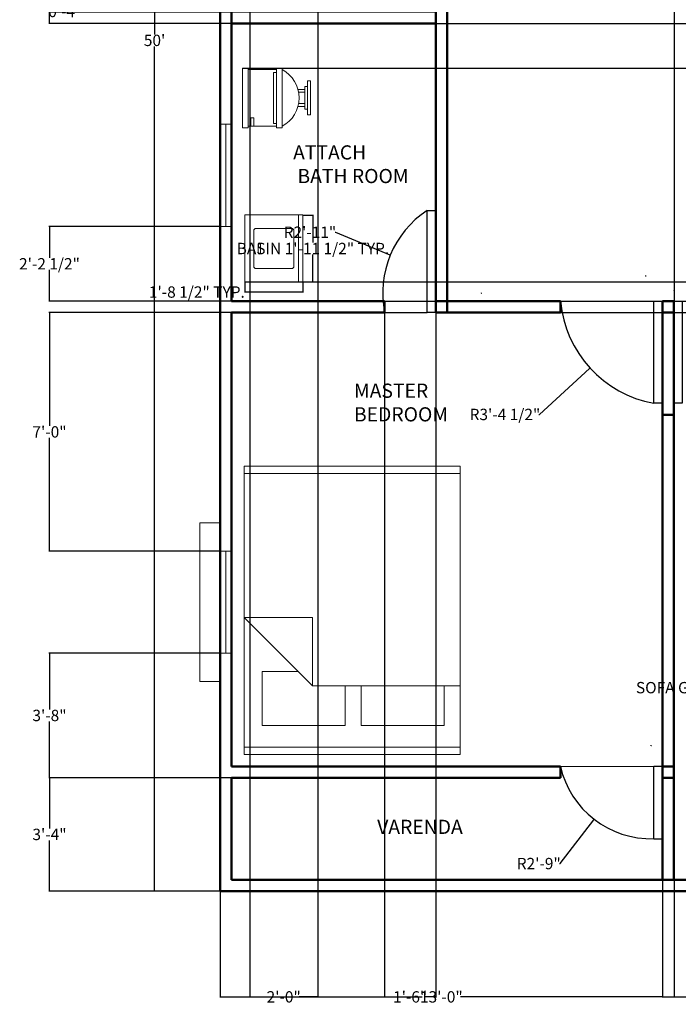
# Model space of a CAD drawing. Units: inches. Extents: x 749 to 1356, y 222 to 907.
# Tile 1 of 4: x 750 to 982, y 222 to 570. Entities that reach past the tile are written whole.
import ezdxf

# ---------------------------------------------------------------- set-up
doc = ezdxf.new("R2010")
doc.units = ezdxf.units.IN
doc.header["$MEASUREMENT"] = 0
for name, color, linetype, lineweight in [('A-ANNO-DIMS', 30, 'Continuous', 18), ('A-AREA-IDEN', 6, 'Continuous', 25), ('A-FLOR-FIXT', 9, 'Continuous', 18), ('A-GLAZ', 4, 'Continuous', 20), ('A-WALL', 7, 'Continuous', 50), ('DOOR', 4, 'Continuous', 25), ('FURNITURE', 32, 'Continuous', 18)]:
    doc.layers.add(name, color=color, linetype=linetype, lineweight=lineweight)
doc.styles.get("Standard").update_dxf_attribs({"font": 'arial.ttf'})
doc.dimstyles.get("Standard").update_dxf_attribs({"dimtxt": 4, "dimasz": 0.18, "dimexe": 0.18, "dimexo": 0.0625, "dimgap": 0.09, "dimtad": 0, "dimtih": 1, "dimtoh": 1, "dimdec": 0, "dimrnd": 6, "dimzin": 0, "dimdsep": 46, "dimlunit": 3, "dimtxsty": 'Standard', "dimcen": 0.09, "dimadec": 0, "dimazin": 0, "dimtfac": 1, "dimtdec": 0, "dimtofl": 0, "dimtmove": 0, "dimatfit": 3, "dimfxl": 1, "dimtolj": 1, "dimtzin": 0, "dimarcsym": 0})

# ---------------------------------------------------------------- blocks, each defined once
blk = doc.blocks.new('Toilet - Imperial')
for p, q in [((-10, 22), (-10, 12)), ((-10, 21), (-7, 21)), ((-7, 21), (-7, 20)), ((10, 12), (10, 22)), ((-7, 20), (-10, 20)), ((10.5, 12), (-10.5, 12)), ((-10.5, 10), (-10.5, 12)), ((9, 13), (-9, 13)), ((-9, 13), (-9, 12)), ((9, 12), (9, 13)), ((10.5, 12), (10.5, 10)), ((10.5, 10), (-10.5, 10)), ((-3, 4.4065), (-3, 2)), ((-2, 2), (-2, 4.1658)), ((2, 4.1658), (2, 2)), ((3, 2), (3, 4.4065)), ((4, 2), (-4, 2)), ((-4, 2), (-4, 1)), ((4, 1), (4, 2))]:
    blk.add_line(p, q)
for points in [[(10.5, 22), (10.5, 24), (-10.5, 24), (-10.5, 22)], [(6, 0), (6, 1), (-6, 1), (-6, 0)]]:
    blk.add_lwpolyline(points, close=True)
blk.add_arc((0, 15.3333), 11.3333, 208.0725, 331.9275)
blk = doc.blocks.new('QUEEN-00')
for p, q in [((-0.8475, -0.7751), (-0.8475, 0.7489)), ((0.6511, 0.7489), (0.6511, -0.2925)), ((1.0829, 0.7489), (1.0829, -0.7751)), ((0.9305, 0.6346), (0.6511, 0.6346)), ((0.9305, 0.0504), (0.9305, 0.6346)), ((0.6511, 0.0504), (0.9305, 0.0504)), ((0.9305, -0.0639), (0.6511, -0.0639)), ((0.9305, -0.6481), (0.9305, -0.0639)), ((0.1685, -0.7751), (0.6511, -0.2925)), ((0.1685, -0.2925), (0.1685, -0.7751)), ((0.6511, -0.2925), (0.1685, -0.2925)), ((0.5495, -0.3941), (0.5495, -0.6481)), ((0.5495, -0.6481), (0.9305, -0.6481))]:
    blk.add_line(p, q)
blk.add_lwpolyline([(-0.8983, -0.7751), (-0.8983, 0.7489), (1.1337, 0.7489), (1.1337, -0.7751)], close=True)
blk = doc.blocks.new('LAVAD-01')
for p, q in [((-0.322, 0.358), (-0.322, -0.392)), ((0.328, 0.358), (-0.322, 0.358)), ((-0.272, 0.358), (-0.272, -0.392)), ((0.328, -0.392), (0.328, 0.358)), ((-0.222, 0.183), (-0.222, -0.217)), ((0.203, 0.208), (-0.197, 0.208)), ((0.228, -0.217), (0.228, 0.183)), ((0.153, 0.033), (0.153, -0.067)), ((0.165, 0.046), (0.165, 0.046)), ((0.178, -0.067), (0.178, 0.033)), ((0.165, -0.079), (0.165, -0.079)), ((-0.197, -0.242), (0.203, -0.242)), ((-0.322, -0.392), (0.328, -0.392))]:
    blk.add_line(p, q)
for centre, radius, start, end in [((-0.197, 0.183), 0.025, 90, 180), ((0.203, 0.183), 0.025, 0, 90), ((0.165, 0.033), 0.0125, 90, 180), ((0.165, 0.033), 0.0125, 0, 90), ((0.165, -0.067), 0.0125, 180, 270), ((0.165, -0.067), 0.0125, 270, 360), ((-0.197, -0.217), 0.025, 180, 270), ((0.203, -0.217), 0.025, 270, 360)]:
    blk.add_arc(centre, radius, start, end)
blk = doc.blocks.new('*D130')
at = {"layer": 'A-ANNO-DIMS', "color": 0, "lineweight": -2, "transparency": 16777216}
for p, q in [((820.81, 862.27), (797.55, 862.27)), ((797.73, 862.09), (797.73, 564.4)), ((797.73, 262.45), (797.73, 560.13)), ((820.81, 262.27), (797.55, 262.27))]:
    blk.add_line(p, q, dxfattribs=at)
at = {"layer": 'A-ANNO-DIMS', "color": 0, "transparency": 16777216}
for points in [[(797.7, 862.09), (797.76, 862.09), (797.73, 862.27)], [(797.7, 262.45), (797.76, 262.45), (797.73, 262.27)]]:
    blk.add_solid(points, dxfattribs=at)
at = {"layer": 'Defpoints', "color": 0, "transparency": 16777216}
for p in [(820.88, 862.27), (797.73, 262.27), (820.88, 262.27)]:
    blk.add_point(p, dxfattribs=at)
at = {"layer": 'A-ANNO-DIMS', "color": 0, "transparency": 16777216, "insert": (797.73, 562.27), "char_height": 4, "attachment_point": 5}
blk.add_mtext("\\A1;50'", dxfattribs=at)
blk = doc.blocks.new('WIN-36IN')
blk.add_lwpolyline([(0, 0), (0, 36), (4, 36), (4, 0)], close=True)
blk.add_lwpolyline([(4, 0), (2.02, 0), (2.02, 36)])
blk = doc.blocks.new('DOOR-LEAF-36IN')
blk.add_lwpolyline([(0, 3), (36, 3), (36, 0), (0, 0)], close=True)
blk = doc.blocks.new('*D143')
at = {"layer": 'A-ANNO-DIMS', "color": 0, "lineweight": -2, "transparency": 16777216}
for p, q in [((850.11, 500.69), (853.77, 500.69)), ((853.59, 500.51), (853.59, 491.04)), ((853.59, 477.25), (853.59, 486.72)), ((850.11, 477.07), (853.77, 477.07))]:
    blk.add_line(p, q, dxfattribs=at)
at = {"layer": 'A-ANNO-DIMS', "color": 0, "transparency": 16777216}
for points in [[(853.56, 500.51), (853.62, 500.51), (853.59, 500.69)], [(853.56, 477.25), (853.62, 477.25), (853.59, 477.07)]]:
    blk.add_solid(points, dxfattribs=at)
at = {"layer": 'Defpoints', "color": 0, "transparency": 16777216}
for p in [(850.05, 500.69), (850.05, 477.07), (853.59, 477.07)]:
    blk.add_point(p, dxfattribs=at)
at = {"layer": 'A-ANNO-DIMS', "color": 0, "transparency": 16777216, "insert": (853.59, 488.88), "char_height": 4, "attachment_point": 5}
blk.add_mtext('\\A1;BASIN 1\'-11 1/2" TYP.', dxfattribs=at)
blk = doc.blocks.new('*D144')
at = {"layer": 'A-ANNO-DIMS', "color": 0, "lineweight": -2, "transparency": 16777216}
for p, q in [((829.57, 477.01), (829.57, 473.35)), ((850.05, 477.01), (850.05, 473.35)), ((829.57, 473.53), (829.39, 473.53)), ((849.87, 473.53), (829.75, 473.53))]:
    blk.add_line(p, q, dxfattribs=at)
at = {"layer": 'A-ANNO-DIMS', "color": 0, "transparency": 16777216}
for points in [[(829.75, 473.56), (829.75, 473.5), (829.57, 473.53)], [(849.87, 473.56), (849.87, 473.5), (850.05, 473.53)]]:
    blk.add_solid(points, dxfattribs=at)
at = {"layer": 'Defpoints', "color": 0, "transparency": 16777216}
for p in [(829.57, 477.07), (850.05, 477.07), (829.57, 473.53)]:
    blk.add_point(p, dxfattribs=at)
at = {"layer": 'A-ANNO-DIMS', "color": 0, "transparency": 16777216, "insert": (812.64, 473.53), "char_height": 4, "attachment_point": 5}
blk.add_mtext('\\A1;1\'-8 1/2" TYP.', dxfattribs=at)
blk = doc.blocks.new('*D153')
at = {"layer": 'A-ANNO-DIMS', "color": 0, "lineweight": -2, "transparency": 16777216}
for p, q in [((1011.97, 388.69), (995.45, 388.69)), ((995.63, 388.51), (995.63, 336.18)), ((995.63, 279.54), (995.63, 331.87)), ((1011.97, 279.36), (995.45, 279.36))]:
    blk.add_line(p, q, dxfattribs=at)
at = {"layer": 'A-ANNO-DIMS', "color": 0, "transparency": 16777216}
for points in [[(995.6, 388.51), (995.66, 388.51), (995.63, 388.69)], [(995.6, 279.54), (995.66, 279.54), (995.63, 279.36)]]:
    blk.add_solid(points, dxfattribs=at)
at = {"layer": 'Defpoints', "color": 0, "transparency": 16777216}
for p in [(1012.03, 388.69), (995.63, 279.36), (1012.03, 279.36)]:
    blk.add_point(p, dxfattribs=at)
at = {"layer": 'A-ANNO-DIMS', "color": 0, "transparency": 16777216, "insert": (995.63, 334.02), "char_height": 4, "attachment_point": 5}
blk.add_mtext('\\A1;SOFA GROUP 9\'-1 1/2"', dxfattribs=at)
blk = doc.blocks.new('*D155')
at = {"layer": 'A-ANNO-DIMS', "color": 0, "lineweight": -2, "transparency": 16777216}
for p, q in [((976.88, 266.2), (976.88, 224.8)), ((820.88, 262.2), (820.88, 224.8)), ((821.06, 224.98), (892.1, 224.98)), ((976.7, 224.98), (905.65, 224.98))]:
    blk.add_line(p, q, dxfattribs=at)
at = {"layer": 'A-ANNO-DIMS', "color": 0, "transparency": 16777216}
for points in [[(821.06, 225.01), (821.06, 224.95), (820.88, 224.98)], [(976.7, 225.01), (976.7, 224.95), (976.88, 224.98)]]:
    blk.add_solid(points, dxfattribs=at)
at = {"layer": 'Defpoints', "color": 0, "transparency": 16777216}
for p in [(976.88, 266.27), (820.88, 262.27), (976.88, 224.98)]:
    blk.add_point(p, dxfattribs=at)
at = {"layer": 'A-ANNO-DIMS', "color": 0, "transparency": 16777216, "insert": (898.88, 224.98), "char_height": 4, "attachment_point": 5}
blk.add_mtext('\\A1;13\'-0"', dxfattribs=at)
blk = doc.blocks.new('*D156')
at = {"layer": 'A-ANNO-DIMS', "color": 0, "lineweight": -2, "transparency": 16777216}
for p, q in [((976.88, 266.2), (976.88, 224.8)), ((1027.01, 266.19), (1027.01, 224.8)), ((977.06, 224.98), (996.46, 224.98)), ((1026.83, 224.98), (1007.43, 224.98))]:
    blk.add_line(p, q, dxfattribs=at)
at = {"layer": 'A-ANNO-DIMS', "color": 0, "transparency": 16777216}
for points in [[(977.06, 225.01), (977.06, 224.95), (976.88, 224.98)], [(1026.83, 225.01), (1026.83, 224.95), (1027.01, 224.98)]]:
    blk.add_solid(points, dxfattribs=at)
at = {"layer": 'Defpoints', "color": 0, "transparency": 16777216}
for p in [(976.88, 266.27), (1027.01, 266.25), (1027.01, 224.98)]:
    blk.add_point(p, dxfattribs=at)
at = {"layer": 'A-ANNO-DIMS', "color": 0, "transparency": 16777216, "insert": (1001.95, 224.98), "char_height": 4, "attachment_point": 5}
blk.add_mtext('\\A1;4\'-2"', dxfattribs=at)
blk = doc.blocks.new('*D159')
at = {"layer": 'A-ANNO-DIMS', "color": 0, "lineweight": -2, "transparency": 16777216}
for p, q in [((824.81, 302.27), (760.48, 302.27)), ((760.66, 302.09), (760.66, 284.4)), ((760.66, 262.45), (760.66, 280.13)), ((820.81, 262.27), (760.48, 262.27))]:
    blk.add_line(p, q, dxfattribs=at)
at = {"layer": 'A-ANNO-DIMS', "color": 0, "transparency": 16777216}
for points in [[(760.63, 302.09), (760.69, 302.09), (760.66, 302.27)], [(760.63, 262.45), (760.69, 262.45), (760.66, 262.27)]]:
    blk.add_solid(points, dxfattribs=at)
at = {"layer": 'Defpoints', "color": 0, "transparency": 16777216}
for p in [(760.66, 302.27), (824.88, 302.27), (820.88, 262.27)]:
    blk.add_point(p, dxfattribs=at)
at = {"layer": 'A-ANNO-DIMS', "color": 0, "transparency": 16777216, "insert": (760.66, 282.27), "char_height": 4, "attachment_point": 5}
blk.add_mtext('\\A1;3\'-4"', dxfattribs=at)
blk = doc.blocks.new('*D160')
at = {"layer": 'A-ANNO-DIMS', "color": 0, "lineweight": -2, "transparency": 16777216}
for p, q in [((820.79, 346.16), (760.48, 346.16)), ((760.66, 345.98), (760.66, 326.35)), ((760.66, 302.45), (760.66, 322.08)), ((824.81, 302.27), (760.48, 302.27))]:
    blk.add_line(p, q, dxfattribs=at)
at = {"layer": 'A-ANNO-DIMS', "color": 0, "transparency": 16777216}
for points in [[(760.63, 345.98), (760.69, 345.98), (760.66, 346.16)], [(760.63, 302.45), (760.69, 302.45), (760.66, 302.27)]]:
    blk.add_solid(points, dxfattribs=at)
at = {"layer": 'Defpoints', "color": 0, "transparency": 16777216}
for p in [(760.66, 346.16), (820.85, 346.16), (824.88, 302.27)]:
    blk.add_point(p, dxfattribs=at)
at = {"layer": 'A-ANNO-DIMS', "color": 0, "transparency": 16777216, "insert": (760.66, 324.21), "char_height": 4, "attachment_point": 5}
blk.add_mtext('\\A1;3\'-8"', dxfattribs=at)
blk = doc.blocks.new('*D161')
at = {"layer": 'A-ANNO-DIMS', "color": 0, "lineweight": -2, "transparency": 16777216}
for p, q in [((824.81, 466.27), (760.48, 466.27)), ((760.66, 466.09), (760.66, 426.35)), ((760.66, 382.34), (760.66, 422.08)), ((820.79, 382.16), (760.48, 382.16))]:
    blk.add_line(p, q, dxfattribs=at)
at = {"layer": 'A-ANNO-DIMS', "color": 0, "transparency": 16777216}
for points in [[(760.63, 466.09), (760.69, 466.09), (760.66, 466.27)], [(760.63, 382.34), (760.69, 382.34), (760.66, 382.16)]]:
    blk.add_solid(points, dxfattribs=at)
at = {"layer": 'Defpoints', "color": 0, "transparency": 16777216}
for p in [(760.66, 466.27), (824.88, 466.27), (820.85, 382.16)]:
    blk.add_point(p, dxfattribs=at)
at = {"layer": 'A-ANNO-DIMS', "color": 0, "transparency": 16777216, "insert": (760.66, 424.21), "char_height": 4, "attachment_point": 5}
blk.add_mtext('\\A1;7\'-0"', dxfattribs=at)
blk = doc.blocks.new('*D170')
at = {"layer": 'A-ANNO-DIMS', "color": 0, "lineweight": -2, "transparency": 16777216}
for p, q in [((820.74, 496.69), (760.48, 496.69)), ((760.66, 496.51), (760.66, 485.63)), ((760.66, 470.45), (760.66, 481.32)), ((824.81, 470.27), (760.48, 470.27))]:
    blk.add_line(p, q, dxfattribs=at)
at = {"layer": 'A-ANNO-DIMS', "color": 0, "transparency": 16777216}
for points in [[(760.63, 496.51), (760.69, 496.51), (760.66, 496.69)], [(760.63, 470.45), (760.69, 470.45), (760.66, 470.27)]]:
    blk.add_solid(points, dxfattribs=at)
at = {"layer": 'Defpoints', "color": 0, "transparency": 16777216}
for p in [(760.66, 496.69), (820.8, 496.69), (824.88, 470.27)]:
    blk.add_point(p, dxfattribs=at)
at = {"layer": 'A-ANNO-DIMS', "color": 0, "transparency": 16777216, "insert": (760.66, 483.48), "char_height": 4, "attachment_point": 5}
blk.add_mtext('\\A1;2\'-2 1/2"', dxfattribs=at)
blk = doc.blocks.new('*D173')
at = {"layer": 'A-ANNO-DIMS', "color": 0, "lineweight": -2, "transparency": 16777216}
for p, q in [((896.94, 568.27), (1340.58, 568.27)), ((1340.4, 568.09), (1340.4, 519.4)), ((1340.4, 466.45), (1340.4, 515.13)), ((900.94, 466.27), (1340.58, 466.27))]:
    blk.add_line(p, q, dxfattribs=at)
at = {"layer": 'A-ANNO-DIMS', "color": 0, "transparency": 16777216}
for points in [[(1340.37, 568.09), (1340.43, 568.09), (1340.4, 568.27)], [(1340.37, 466.45), (1340.43, 466.45), (1340.4, 466.27)]]:
    blk.add_solid(points, dxfattribs=at)
at = {"layer": 'Defpoints', "color": 0, "transparency": 16777216}
for p in [(896.88, 568.27), (1340.4, 568.27), (900.88, 466.27)]:
    blk.add_point(p, dxfattribs=at)
at = {"layer": 'A-ANNO-DIMS', "color": 0, "transparency": 16777216, "insert": (1340.4, 517.27), "char_height": 4, "attachment_point": 5}
blk.add_mtext('\\A1;8\'-6"', dxfattribs=at)
blk = doc.blocks.new('*D176')
at = {"layer": 'A-ANNO-DIMS', "color": 0, "lineweight": -2, "transparency": 16777216}
for p, q in [((878.88, 466.2), (878.88, 224.8)), ((896.88, 466.2), (896.88, 224.8)), ((879.06, 224.98), (882.66, 224.98)), ((896.7, 224.98), (893.1, 224.98))]:
    blk.add_line(p, q, dxfattribs=at)
at = {"layer": 'A-ANNO-DIMS', "color": 0, "transparency": 16777216}
for points in [[(879.06, 225.01), (879.06, 224.95), (878.88, 224.98)], [(896.7, 225.01), (896.7, 224.95), (896.88, 224.98)]]:
    blk.add_solid(points, dxfattribs=at)
at = {"layer": 'Defpoints', "color": 0, "transparency": 16777216}
for p in [(878.88, 466.27), (896.88, 466.27), (896.88, 224.98)]:
    blk.add_point(p, dxfattribs=at)
at = {"layer": 'A-ANNO-DIMS', "color": 0, "transparency": 16777216, "insert": (887.88, 224.98), "char_height": 4, "attachment_point": 5}
blk.add_mtext('\\A1;1\'-6"', dxfattribs=at)
blk = doc.blocks.new('*D177')
at = {"layer": 'A-ANNO-DIMS', "color": 0, "lineweight": -2, "transparency": 16777216}
for p, q in [((855.27, 592.42), (855.27, 224.8)), ((831.27, 587.92), (831.27, 224.8)), ((831.45, 224.98), (837.83, 224.98)), ((855.09, 224.98), (848.71, 224.98))]:
    blk.add_line(p, q, dxfattribs=at)
at = {"layer": 'A-ANNO-DIMS', "color": 0, "transparency": 16777216}
for points in [[(831.45, 225.01), (831.45, 224.95), (831.27, 224.98)], [(855.09, 225.01), (855.09, 224.95), (855.27, 224.98)]]:
    blk.add_solid(points, dxfattribs=at)
at = {"layer": 'Defpoints', "color": 0, "transparency": 16777216}
for p in [(855.27, 592.48), (831.27, 587.98), (855.27, 224.98)]:
    blk.add_point(p, dxfattribs=at)
at = {"layer": 'A-ANNO-DIMS', "color": 0, "transparency": 16777216, "insert": (843.27, 224.98), "char_height": 4, "attachment_point": 5}
blk.add_mtext('\\A1;2\'-0"', dxfattribs=at)
blk = doc.blocks.new('*D180')
at = {"layer": 'A-ANNO-DIMS', "color": 0, "lineweight": -2, "transparency": 16777216}
for p, q in [((980.98, 762.26), (980.98, 224.8)), ((1132.88, 762.2), (1132.88, 224.8)), ((981.16, 224.98), (1050.16, 224.98)), ((1132.7, 224.98), (1063.7, 224.98))]:
    blk.add_line(p, q, dxfattribs=at)
at = {"layer": 'A-ANNO-DIMS', "color": 0, "transparency": 16777216}
for points in [[(981.16, 225.01), (981.16, 224.95), (980.98, 224.98)], [(1132.7, 225.01), (1132.7, 224.95), (1132.88, 224.98)]]:
    blk.add_solid(points, dxfattribs=at)
at = {"layer": 'Defpoints', "color": 0, "transparency": 16777216}
for p in [(980.98, 762.32), (1132.88, 762.27), (1132.88, 224.98)]:
    blk.add_point(p, dxfattribs=at)
at = {"layer": 'A-ANNO-DIMS', "color": 0, "transparency": 16777216, "insert": (1056.93, 224.98), "char_height": 4, "attachment_point": 5}
blk.add_mtext('\\A1;12\'-8"', dxfattribs=at)
blk = doc.blocks.new('*D183')
at = {"layer": 'A-ANNO-DIMS', "color": 0, "lineweight": -2, "transparency": 16777216}
for p, q in [((896.81, 572.27), (760.48, 572.27)), ((760.66, 572.27), (760.66, 572.45)), ((760.66, 572.45), (760.84, 572.45)), ((760.66, 568.45), (760.66, 572.09)), ((896.81, 568.27), (760.48, 568.27))]:
    blk.add_line(p, q, dxfattribs=at)
at = {"layer": 'A-ANNO-DIMS', "color": 0, "transparency": 16777216}
for points in [[(760.63, 572.09), (760.69, 572.09), (760.66, 572.27)], [(760.63, 568.45), (760.69, 568.45), (760.66, 568.27)]]:
    blk.add_solid(points, dxfattribs=at)
at = {"layer": 'Defpoints', "color": 0, "transparency": 16777216}
for p in [(760.66, 572.27), (896.88, 572.27), (896.88, 568.27)]:
    blk.add_point(p, dxfattribs=at)
at = {"layer": 'A-ANNO-DIMS', "color": 0, "transparency": 16777216, "insert": (766.25, 572.45), "char_height": 4, "attachment_point": 5}
blk.add_mtext('\\A1;0\'-4"', dxfattribs=at)
blk = doc.blocks.new('*D189')
at = {"layer": 'A-ANNO-DIMS', "color": 0, "lineweight": -2, "transparency": 16777216}
for p, q in [((829.64, 477.07), (1340.58, 477.07)), ((1340.4, 476.89), (1340.4, 475.8)), ((824.94, 470.27), (1340.58, 470.27)), ((1340.4, 470.45), (1340.4, 471.54))]:
    blk.add_line(p, q, dxfattribs=at)
at = {"layer": 'A-ANNO-DIMS', "color": 0, "transparency": 16777216}
for points in [[(1340.37, 476.89), (1340.43, 476.89), (1340.4, 477.07)], [(1340.37, 470.45), (1340.43, 470.45), (1340.4, 470.27)]]:
    blk.add_solid(points, dxfattribs=at)
at = {"layer": 'Defpoints', "color": 0, "transparency": 16777216}
for p in [(829.57, 477.07), (824.88, 470.27), (1340.4, 470.27)]:
    blk.add_point(p, dxfattribs=at)
at = {"layer": 'A-ANNO-DIMS', "color": 0, "transparency": 16777216, "insert": (1340.4, 473.67), "char_height": 4, "attachment_point": 5}
blk.add_mtext('\\A1;0\'-7"', dxfattribs=at)
blk = doc.blocks.new('*D190')
at = {"layer": 'A-ANNO-DIMS', "color": 0, "lineweight": -2, "transparency": 16777216}
for p, q in [((824.94, 568.27), (1340.58, 568.27)), ((1340.4, 568.09), (1340.4, 562.47)), ((1340.4, 552.65), (1340.4, 558.27)), ((828.78, 552.47), (1340.58, 552.47))]:
    blk.add_line(p, q, dxfattribs=at)
at = {"layer": 'A-ANNO-DIMS', "color": 0, "transparency": 16777216}
for points in [[(1340.37, 568.09), (1340.43, 568.09), (1340.4, 568.27)], [(1340.37, 552.65), (1340.43, 552.65), (1340.4, 552.47)]]:
    blk.add_solid(points, dxfattribs=at)
at = {"layer": 'Defpoints', "color": 0, "transparency": 16777216}
for p in [(824.88, 568.27), (1340.4, 568.27), (828.71, 552.47)]:
    blk.add_point(p, dxfattribs=at)
at = {"layer": 'A-ANNO-DIMS', "color": 0, "transparency": 16777216, "insert": (1340.4, 560.37), "char_height": 4, "attachment_point": 5}
blk.add_mtext('\\A1;1\'-4"', dxfattribs=at)
blk = doc.blocks.new('*D191')
at = {"layer": 'A-ANNO-DIMS', "color": 0, "lineweight": -2, "transparency": 16777216}
for p, q in [((970.9, 479.27), (971.08, 479.27)), ((970.99, 479.18), (970.99, 479.36)), ((1026.07, 428.63), (1005.55, 447.5)), ((1026.25, 428.63), (1026.07, 428.63))]:
    blk.add_line(p, q, dxfattribs=at)
at = {"layer": 'A-ANNO-DIMS', "color": 0, "transparency": 16777216}
blk.add_solid([(1005.57, 447.52), (1005.53, 447.47), (1005.41, 447.62)], dxfattribs=at)
at = {"layer": 'Defpoints', "color": 0, "transparency": 16777216}
for p in [(970.99, 479.27), (1005.41, 447.62)]:
    blk.add_point(p, dxfattribs=at)
at = {"layer": 'A-ANNO-DIMS', "color": 0, "transparency": 16777216, "insert": (1035.12, 428.63), "char_height": 4, "attachment_point": 5}
blk.add_mtext('\\A1;R3\'-11"', dxfattribs=at)
blk = doc.blocks.new('*D193')
at = {"layer": 'A-ANNO-DIMS', "color": 0, "lineweight": -2, "transparency": 16777216}
for p, q in [((980.95, 473.99), (981.13, 473.99)), ((981.04, 473.9), (981.04, 474.08)), ((933.48, 430.36), (951.18, 446.6)), ((933.3, 430.36), (933.48, 430.36))]:
    blk.add_line(p, q, dxfattribs=at)
at = {"layer": 'A-ANNO-DIMS', "color": 0, "transparency": 16777216}
blk.add_solid([(951.16, 446.62), (951.2, 446.58), (951.32, 446.72)], dxfattribs=at)
at = {"layer": 'Defpoints', "color": 0, "transparency": 16777216}
for p in [(981.04, 473.99), (951.32, 446.72)]:
    blk.add_point(p, dxfattribs=at)
at = {"layer": 'A-ANNO-DIMS', "color": 0, "transparency": 16777216, "insert": (921.32, 430.36), "char_height": 4, "attachment_point": 5}
blk.add_mtext('\\A1;R3\'-4 1/2"', dxfattribs=at)
blk = doc.blocks.new('*D196')
at = {"layer": 'A-ANNO-DIMS', "color": 0, "lineweight": -2, "transparency": 16777216}
for p, q in [((861.39, 494.61), (861.57, 494.61)), ((861.57, 494.61), (880.69, 486.64)), ((912.92, 473.18), (913.1, 473.18)), ((913.01, 473.09), (913.01, 473.27))]:
    blk.add_line(p, q, dxfattribs=at)
at = {"layer": 'A-ANNO-DIMS', "color": 0, "transparency": 16777216}
blk.add_solid([(880.71, 486.67), (880.68, 486.61), (880.86, 486.57)], dxfattribs=at)
at = {"layer": 'Defpoints', "color": 0, "transparency": 16777216}
for p in [(880.86, 486.57), (913.01, 473.18)]:
    blk.add_point(p, dxfattribs=at)
at = {"layer": 'A-ANNO-DIMS', "color": 0, "transparency": 16777216, "insert": (852.52, 494.61), "char_height": 4, "attachment_point": 5}
blk.add_mtext('\\A1;R2\'-11"', dxfattribs=at)
blk = doc.blocks.new('*D198')
at = {"layer": 'A-ANNO-DIMS', "color": 0, "lineweight": -2, "transparency": 16777216}
for p, q in [((972.84, 313.6), (973.02, 313.6)), ((972.93, 313.51), (972.93, 313.69)), ((940.74, 271.99), (952.7, 287.45)), ((940.56, 271.99), (940.74, 271.99))]:
    blk.add_line(p, q, dxfattribs=at)
at = {"layer": 'A-ANNO-DIMS', "color": 0, "transparency": 16777216}
blk.add_solid([(952.68, 287.47), (952.72, 287.44), (952.81, 287.6)], dxfattribs=at)
at = {"layer": 'Defpoints', "color": 0, "transparency": 16777216}
for p in [(972.93, 313.6), (952.81, 287.6)]:
    blk.add_point(p, dxfattribs=at)
at = {"layer": 'A-ANNO-DIMS', "color": 0, "transparency": 16777216, "insert": (933.24, 271.99), "char_height": 4, "attachment_point": 5}
blk.add_mtext('\\A1;R2\'-9"', dxfattribs=at)

msp = doc.modelspace()

# ---------------------------------------------------------------- linework, layer by layer
at = {"layer": 'A-GLAZ'}
for p, q in [((813.64, 392.16), (820.88, 392.16)), ((813.64, 336.16), (813.64, 392.16)), ((813.64, 336.16), (820.88, 336.16))]:
    msp.add_line(p, q, dxfattribs=at)
at = {"layer": 'A-WALL'}
for p, q in [((820.88, 862.27), (820.88, 262.27)), ((824.88, 818.27), (824.88, 470.27)), ((900.88, 646.27), (900.88, 466.27)), ((896.88, 572.27), (896.88, 568.27)), ((896.88, 568.27), (824.88, 568.27)), ((896.88, 568.27), (896.88, 466.27)), ((878.88, 470.27), (824.88, 470.27)), ((878.88, 470.27), (878.88, 466.27)), ((940.88, 470.27), (896.88, 470.27)), ((940.88, 470.27), (940.88, 466.27)), ((976.88, 470.27), (976.88, 266.27)), ((980.88, 470.27), (976.88, 470.27)), ((980.88, 470.27), (980.88, 266.27)), ((878.88, 466.27), (824.88, 466.27)), ((824.88, 466.27), (824.88, 306.27)), ((940.88, 466.27), (896.88, 466.27)), ((980.88, 466.27), (976.88, 466.27)), ((980.88, 430.27), (976.88, 430.27)), ((824.88, 306.27), (940.88, 306.27)), ((940.88, 306.27), (940.88, 302.27)), ((976.88, 306.27), (980.88, 306.27)), ((824.88, 302.27), (940.88, 302.27)), ((824.88, 302.27), (824.88, 266.27)), ((976.88, 302.27), (980.88, 302.27)), ((824.88, 266.27), (1132.88, 266.27)), ((820.88, 262.27), (1136.88, 262.27))]:
    msp.add_line(p, q, dxfattribs=at)
at = {"layer": 'DOOR'}
for p, q in [((940.88, 470.27), (976.88, 470.3)), ((878.88, 466.27), (893.88, 466.28)), ((940.88, 306.27), (973.88, 306.3)), ((973.88, 280.74), (976.88, 280.74))]:
    msp.add_line(p, q, dxfattribs=at)
msp.add_lwpolyline([(973.88, 280.74), (973.88, 306.3), (976.88, 306.3), (976.88, 280.74)], dxfattribs=at)
for centre, radius, start, end in [((913.01, 473.18), 34.83, 123.3264, 191.4515), ((981.04, 473.99), 40.33, 185.2942, 259.7716), ((972.93, 313.6), 32.88, 192.8905, 271.6516)]:
    msp.add_arc(centre, radius, start, end, dxfattribs=at)

# ---------------------------------------------------------------- block references
at = {"layer": 'A-FLOR-FIXT', "rotation": 90}
msp.add_blockref('Toilet - Imperial', (852.71, 541.97), dxfattribs=at)
at = {"layer": 'A-FLOR-FIXT', "xscale": 31.49606299212599, "yscale": 31.49606299212599, "zscale": 31.49606299212599, "rotation": 180}
msp.add_blockref('LAVAD-01', (839.9, 488.36), dxfattribs=at)
at = {"layer": 'A-GLAZ'}
for p in [(820.8, 496.69), (820.85, 346.16)]:
    msp.add_blockref('WIN-36IN', p, dxfattribs=at)
at = {"layer": 'DOOR'}
for p, rotation in [((893.88, 502.28), 269.9999999999997), ((973.88, 470.3), 269.9999999999994), ((980.81, 470.3), 270)]:
    msp.add_blockref('DOOR-LEAF-36IN', p, dxfattribs=dict(at, rotation=rotation))
at = {"layer": 'FURNITURE', "xscale": 49.9999999999977, "yscale": 49.9999999999977, "zscale": 49.9999999999977, "rotation": 270}
msp.add_blockref('QUEEN-00', (868.1, 367.17), dxfattribs=at)

# ---------------------------------------------------------------- texts
at = {"layer": 'A-AREA-IDEN', "char_height": 5, "attachment_point": 1}
for s, insert in [('ATTACH\\P BATH ROOM', (846.59, 525.27)), ('MASTER BEDROOM', (868.06, 441.24)), ('VARENDA', (876.25, 287.43))]:
    msp.add_mtext_dynamic_manual_height_columns(s, width=49.3334, gutter_width=1, heights=[0], dxfattribs=dict(at, insert=insert))

# ---------------------------------------------------------------- dimensions: what is measured, and where the dimension line sits
at = {"layer": 'A-ANNO-DIMS'}
for base, p1, p2, override, picture, middle in [((797.73, 262.27), (820.88, 862.27), (820.88, 262.27), {"dimclrd": 0, "dimclre": 0, "dimclrt": 0}, '*D130', (797.73, 562.27)), ((760.66, 572.27), (896.88, 568.27), (896.88, 572.27), {"dimdec": 1, "dimlfac": 1, "dimrnd": 0, "dimzin": 1, "dimdsep": 46, "dimlunit": 4, "dimfrac": 2}, '*D183', (766.25, 572.45)), ((1340.4, 568.27), (828.71, 552.47), (824.88, 568.27), {"dimdec": 1, "dimlfac": 1, "dimrnd": 0, "dimzin": 1, "dimdsep": 46, "dimlunit": 4, "dimfrac": 2}, '*D190', (1340.4, 560.37)), ((1340.4, 568.27), (900.88, 466.27), (896.88, 568.27), {"dimdec": 1, "dimlfac": 1, "dimrnd": 0, "dimzin": 1, "dimdsep": 46, "dimlunit": 4, "dimfrac": 2}, '*D173', (1340.4, 517.27)), ((760.66, 496.69), (824.88, 470.27), (820.8, 496.69), {"dimdec": 1, "dimlfac": 1, "dimrnd": 0, "dimzin": 1, "dimdsep": 46, "dimlunit": 4, "dimfrac": 2}, '*D170', (760.66, 483.48)), ((1340.4, 470.27), (829.57, 477.07), (824.88, 470.27), {"dimdec": 1, "dimlfac": 1, "dimrnd": 0, "dimzin": 1, "dimdsep": 46, "dimlunit": 4, "dimfrac": 2}, '*D189', (1340.4, 473.67)), ((760.66, 466.27), (820.85, 382.16), (824.88, 466.27), {"dimdec": 1, "dimlfac": 1, "dimrnd": 0, "dimzin": 1, "dimdsep": 46, "dimlunit": 4, "dimfrac": 2}, '*D161', (760.66, 424.21)), ((760.66, 346.16), (824.88, 302.27), (820.85, 346.16), {"dimdec": 1, "dimlfac": 1, "dimrnd": 0, "dimzin": 1, "dimdsep": 46, "dimlunit": 4, "dimfrac": 2}, '*D160', (760.66, 324.21)), ((760.66, 302.27), (820.88, 262.27), (824.88, 302.27), {"dimdec": 1, "dimlfac": 1, "dimrnd": 0, "dimzin": 1, "dimdsep": 46, "dimlunit": 4, "dimfrac": 2}, '*D159', (760.66, 282.27))]:
    dim = msp.add_linear_dim(base=base, p1=p1, p2=p2, angle=90, dimstyle='Standard', override=override, dxfattribs=at)
    dim.commit()
    dim.dimension.update_dxf_attribs({"geometry": picture, "text_midpoint": middle})
for base, p1, p2, picture, middle in [((1132.88, 224.98), (980.98, 762.32), (1132.88, 762.27), '*D180', (1056.93, 224.98)), ((855.27, 224.98), (831.27, 587.98), (855.27, 592.48), '*D177', (843.27, 224.98)), ((896.88, 224.98), (878.88, 466.27), (896.88, 466.27), '*D176', (887.88, 224.98)), ((976.88, 224.98), (820.88, 262.27), (976.88, 266.27), '*D155', (898.88, 224.98)), ((1027.01, 224.98), (976.88, 266.27), (1027.01, 266.25), '*D156', (1001.95, 224.98))]:
    dim = msp.add_linear_dim(base=base, p1=p1, p2=p2, dimstyle='Standard', override={"dimdec": 1, "dimlfac": 1, "dimrnd": 0, "dimzin": 1, "dimdsep": 46, "dimlunit": 4, "dimfrac": 2}, dxfattribs=at)
    dim.commit()
    dim.dimension.update_dxf_attribs({"geometry": picture, "text_midpoint": middle})
for base, p1, p2, angle, text, picture, middle in [((853.59, 477.07), (850.05, 500.69), (850.05, 477.07), 270, 'BASIN <> TYP.', '*D143', (853.59, 488.88)), ((829.57, 473.53), (850.05, 477.07), (829.57, 477.07), 180, '<> TYP.', '*D144', (812.64, 473.53)), ((995.63, 279.36), (1012.03, 388.69), (1012.03, 279.36), 270, 'SOFA GROUP <>', '*D153', (995.63, 334.02))]:
    dim = msp.add_linear_dim(base=base, p1=p1, p2=p2, angle=angle, text=text, dimstyle='Standard', override={"dimdec": 1, "dimlfac": 1, "dimrnd": 0, "dimzin": 1, "dimdsep": 46, "dimlunit": 4, "dimfrac": 2}, dxfattribs=at)
    dim.commit()
    dim.dimension.update_dxf_attribs({"geometry": picture, "text_midpoint": middle})
for center, mpoint, picture, middle in [((913.01, 473.18), (880.86, 486.57), '*D196', (852.52, 494.61)), ((970.99, 479.27), (1005.41, 447.62), '*D191', (1035.12, 428.63)), ((981.04, 473.99), (951.32, 446.72), '*D193', (921.32, 430.36)), ((972.93, 313.6), (952.81, 287.6), '*D198', (933.24, 271.99))]:
    dim = msp.add_radius_dim(center=center, mpoint=mpoint, dimstyle='Standard', override={"dimdec": 1, "dimlfac": 1, "dimrnd": 0, "dimzin": 1, "dimdsep": 46, "dimlunit": 4, "dimfrac": 2}, dxfattribs=at)
    dim.commit()
    dim.dimension.update_dxf_attribs({"geometry": picture, "text_midpoint": middle, "dimtype": 164})

doc.saveas('drawing.dxf')
